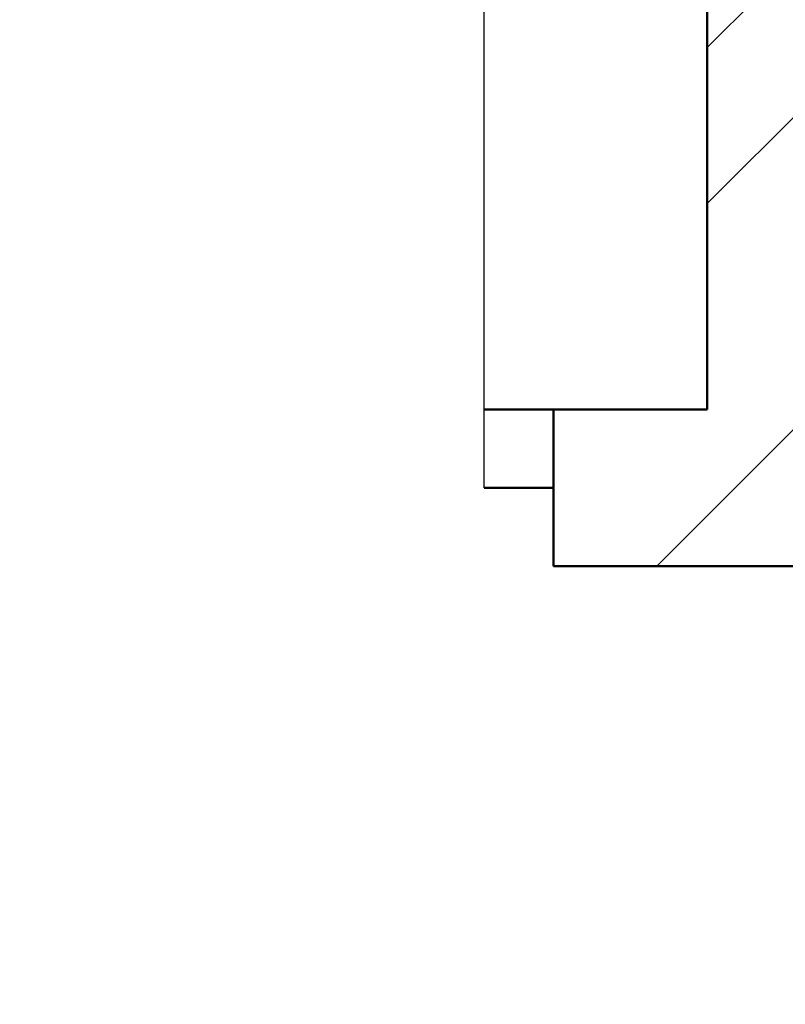
# Model space of a CAD drawing. Units: inches. Extents: x 1901 to 2863, y 888 to 2433.
# Tile 75 of 91: x 2586 to 2608, y 2066 to 2094. Entities that reach past the tile are written whole.
import ezdxf

# ---------------------------------------------------------------- set-up
doc = ezdxf.new("R2010")
doc.units = ezdxf.units.IN
for name, color, linetype, lineweight in [('A-DOOR', 4, 'Continuous', 25), ('A-WALL', 7, 'Continuous', 50), ('A-WALL-PATT', 8, 'Continuous', 13)]:
    doc.layers.add(name, color=color, linetype=linetype, lineweight=lineweight)

# ---------------------------------------------------------------- blocks, each defined once
blk = doc.blocks.new('DOOR-27')
blk.add_line((26.814, -0.016), (26.814, 35.984))
blk.add_arc((26.814, 9.122), 26.862, 90, 199.8893)

msp = doc.modelspace()

# ---------------------------------------------------------------- hatches: boundary and pattern name
at = {"layer": 'A-WALL-PATT'}
h = msp.add_hatch(dxfattribs=at)
h.set_pattern_fill('ANSI32', color=256)
h.paths.add_polyline_path([(2192.501, 2274.134), (2141.264, 2274.134), (2141.264, 2269.634), (2192.501, 2269.634)])
h.paths.add_polyline_path([(2259.926, 2274.134), (2216.501, 2274.134), (2216.501, 2269.634), (2255.426, 2269.634), (2255.426, 2214.634), (2250.809, 2214.634), (2250.809, 2210.134), (2259.926, 2210.134), (2259.926, 2215.134), (2271.756, 2215.134), (2271.756, 2217.384), (2271.756, 2219.634), (2259.926, 2219.634)])
h.paths.add_polyline_path([(2171.426, 2269.634), (2166.926, 2269.634), (2166.926, 2219.634), (2121.238, 2219.634), (2121.238, 2215.134), (2166.926, 2215.134), (2166.926, 2083.134), (2161.807, 2083.134), (2161.807, 2078.634), (2171.426, 2078.634), (2176.996, 2078.634), (2176.996, 2080.884), (2176.996, 2083.134), (2171.426, 2083.134), (2171.426, 2210.134), (2230.912, 2210.134), (2230.912, 2212.384), (2230.912, 2214.634), (2171.426, 2214.634)])
h.paths.add_polyline_path([(2117.264, 2274.134), (2089.426, 2274.134), (2089.426, 2219.634), (2081.136, 2219.634), (2081.136, 2215.134), (2089.426, 2215.134), (2098.004, 2215.134), (2098.004, 2217.384), (2098.004, 2219.634), (2093.926, 2219.634), (2093.926, 2269.634), (2117.264, 2269.634), (2117.264, 2271.884)])
h.paths.add_polyline_path([(2343.426, 2219.634), (2329.295, 2219.634), (2329.295, 2215.134), (2338.926, 2215.134), (2338.926, 2184.739), (2343.426, 2184.739)])
h.paths.add_polyline_path([(2338.926, 2083.134), (2329.295, 2083.134), (2208.966, 2083.134), (2208.966, 2078.634), (2338.926, 2078.634)])
h.paths.add_polyline_path([(2343.426, 2136.739), (2338.926, 2136.739), (2338.926, 1872.634), (2343.426, 1872.634)])
h.paths.add_polyline_path([(2343.426, 1863.634), (2397.68, 1863.634), (2397.68, 1821.634), (2384.138, 1821.634), (2384.138, 1812.634), (2418.33, 1812.634), (2418.33, 1817.134), (2418.33, 1821.634), (2406.68, 1821.634), (2406.68, 1863.634), (2459.499, 1863.634), (2459.499, 1821.634), (2447.138, 1821.634), (2447.138, 1812.634), (2459.499, 1812.634), (2468.499, 1812.634), (2468.499, 1872.634), (2394.426, 1872.634), (2334.426, 1872.634), (2334.426, 1812.634), (2343.426, 1812.634), (2353.251, 1812.634), (2353.251, 1821.634), (2343.426, 1821.634)])
h.paths.add_polyline_path([(2510.014, 1872.634), (2468.499, 1872.634), (2468.499, 1868.134), (2510.014, 1868.134)])
h.paths.add_polyline_path([(2514.009, 1817.134), (2468.499, 1817.134), (2468.499, 1812.634), (2482.114, 1812.634), (2482.114, 1800.606), (2486.614, 1800.606), (2486.614, 1812.634), (2514.009, 1812.634)])
h.paths.add_polyline_path([(2299.247, 1814.884), (2299.247, 1817.134), (2295.926, 1817.134), (2295.926, 1854.169), (2293.676, 1854.169), (2291.426, 1854.169), (2291.426, 1817.134), (2266.109, 1817.134), (2266.109, 1812.634), (2299.247, 1812.634)])
h.paths.add_polyline_path([(2218.109, 1817.134), (2206.46, 1817.134), (2171.426, 1817.134), (2171.426, 1949.134), (2190.1, 1949.134), (2190.1, 1953.634), (2163.468, 1953.634), (2163.468, 1949.134), (2166.926, 1949.134), (2166.926, 1817.134), (2114.297, 1817.134), (2114.297, 1812.634), (2218.109, 1812.634)])
h.paths.add_polyline_path([(2029.426, 1970.922), (2024.926, 1970.922), (2024.926, 1912.717), (2029.426, 1912.717)])
h.paths.add_polyline_path([(2132.297, 1953.634), (2113.926, 1953.634), (2113.926, 1975.888), (2111.676, 1975.888), (2109.426, 1975.888), (2109.426, 1953.634), (2029.426, 1953.634), (2029.426, 1949.134), (2132.297, 1949.134)])
h.paths.add_polyline_path([(2029.426, 1853.606), (2029.31, 1853.606), (2029.31, 1853.606), (2029.426, 1853.606), (2029.426, 1864.717), (2024.926, 1864.717), (2024.926, 1812.634), (2066.297, 1812.634), (2066.297, 1814.884), (2066.297, 1817.134), (2029.426, 1817.134)])
h.paths.add_polyline_path([(2122.926, 2010.088), (2120.676, 2010.088), (2118.426, 2010.088), (2118.426, 2006.134), (2029.426, 2006.134), (2029.426, 2001.634), (2109.426, 2001.634), (2109.426, 1998.041), (2113.926, 1998.041), (2113.926, 2001.634), (2122.926, 2001.634)])
h.paths.add_polyline_path([(2029.426, 2031.376), (2024.926, 2031.376), (2024.926, 1994.922), (2027.176, 1994.922), (2029.426, 1994.922)])
h.paths.add_polyline_path([(2029.426, 2136.739), (2024.926, 2136.739), (2024.926, 2067.376), (2027.176, 2067.376), (2029.426, 2067.376)])
h.paths.add_polyline_path([(2125.618, 2083.134), (2029.426, 2083.134), (2029.426, 2078.634), (2118.426, 2078.634), (2118.426, 2030.715), (2122.926, 2030.715), (2122.926, 2078.634), (2125.618, 2078.634)])
h.paths.add_polyline_path([(2029.426, 2215.134), (2040.468, 2215.134), (2040.468, 2217.384), (2040.468, 2219.634), (2024.926, 2219.634), (2024.926, 2184.739), (2029.426, 2184.739), (2029.426, 2187.778)])
h.paths.add_polyline_path([(2686.426, 2274.134), (2659.284, 2274.134), (2659.284, 2269.634), (2681.926, 2269.634), (2681.926, 2219.634), (2676.816, 2219.634), (2676.816, 2215.134), (2681.926, 2215.134), (2697.011, 2215.134), (2697.011, 2217.384), (2697.011, 2219.634), (2686.426, 2219.634)])
h.paths.add_polyline_path([(2609.926, 2269.634), (2635.284, 2269.634), (2635.284, 2274.134), (2571.431, 2274.134), (2571.431, 2269.634), (2605.426, 2269.634), (2605.426, 2214.634), (2549.098, 2214.634), (2549.098, 2210.134), (2605.426, 2210.134), (2605.426, 2083.134), (2601.014, 2083.134), (2601.014, 2080.884), (2601.014, 2078.634), (2609.926, 2078.634), (2616.162, 2078.634), (2616.162, 2080.884), (2616.162, 2083.134), (2609.926, 2083.134), (2609.926, 2215.134), (2651.465, 2215.134), (2651.465, 2217.384), (2651.465, 2219.634), (2609.926, 2219.634)])
h.paths.add_polyline_path([(2521.426, 2269.634), (2547.431, 2269.634), (2547.431, 2271.884), (2547.431, 2274.134), (2516.926, 2274.134), (2516.926, 2219.634), (2506.41, 2219.634), (2506.41, 2215.134), (2516.926, 2215.134), (2516.926, 2210.134), (2525.402, 2210.134), (2525.402, 2212.384), (2525.402, 2214.634), (2521.426, 2214.634)])
h.paths.add_polyline_path([(2456.011, 2219.634), (2439.426, 2219.634), (2439.426, 2187.888), (2443.926, 2187.888), (2443.926, 2215.134), (2456.011, 2215.134)])
h.paths.add_polyline_path([(2752.926, 2219.634), (2739.485, 2219.634), (2739.485, 2215.134), (2748.426, 2215.134), (2748.426, 2187.888), (2752.926, 2187.888)])
h.paths.add_polyline_path([(2752.926, 2139.888), (2748.426, 2139.888), (2748.426, 2083.134), (2648.416, 2083.134), (2648.416, 2078.634), (2654.926, 2078.634), (2654.926, 2039.437), (2659.426, 2039.437), (2659.426, 2078.634), (2748.426, 2078.634), (2748.426, 2063.429), (2752.926, 2063.429)])
h.paths.add_polyline_path([(2752.926, 2010.634), (2659.426, 2010.634), (2659.426, 2015.652), (2654.926, 2015.652), (2654.926, 2010.634), (2605.426, 2010.634), (2605.426, 1920.967), (2609.926, 1920.967), (2609.926, 2006.134), (2748.426, 2006.134), (2748.426, 1982.466), (2752.926, 1982.466)])
h.paths.add_polyline_path([(2752.926, 2027.429), (2748.426, 2027.429), (2748.426, 2010.634), (2752.926, 2010.634)])
h.paths.add_polyline_path([(2748.426, 1886.134), (2609.926, 1886.134), (2609.926, 1889.719), (2605.426, 1889.719), (2605.426, 1861.262), (2609.926, 1861.262), (2609.926, 1881.634), (2748.426, 1881.634)])
h.paths.add_polyline_path([(2456.855, 2228.831), (2498.401, 2228.831), (2498.401, 2247.488), (2456.855, 2247.488)], flags=9)
h.paths.add_polyline_path([(2038.602, 2237.418), (2080.174, 2237.418), (2080.174, 2256.075), (2038.602, 2256.075)], flags=9)
h.paths.add_polyline_path([(2292.009, 1062.394), (2539.932, 1062.394), (2539.932, 1099.487), (2292.009, 1099.487)], flags=9)
h.paths.add_polyline_path([(2424.91, 1832.253), (2448.513, 1832.253), (2448.513, 1846.678), (2424.91, 1846.678)], flags=25)
h.paths.add_polyline_path([(2359.076, 1832.253), (2382.678, 1832.253), (2382.678, 1846.678), (2359.076, 1846.678)], flags=25)
h.paths.add_polyline_path([(2352.899, 1684.802), (2367.543, 1684.802), (2367.543, 1697.167), (2352.899, 1697.167)], flags=9)
h.paths.add_polyline_path([(2079.288, 1755.826), (2169.024, 1755.826), (2169.024, 1774.372), (2079.288, 1774.372)], flags=9)
h.paths.add_polyline_path([(2404.09, 1373.857), (2404.09, 1463.593), (2385.544, 1463.593), (2385.544, 1373.857)], flags=9)
h.paths.add_polyline_path([(2268.091, 2236.371), (2309.636, 2236.371), (2309.636, 2255.028), (2268.091, 2255.028)], flags=9)
h.paths.add_polyline_path([(2575.96, 1700.951), (2665.696, 1700.951), (2665.696, 1719.498), (2575.96, 1719.498)], flags=9)
h.paths.add_polyline_path([(2302.962, 1878.474), (2329.524, 1878.474), (2329.524, 1888.777), (2302.962, 1888.777)], flags=9)
h.paths.add_polyline_path([(2097.415, 2240.576), (2126.573, 2240.576), (2126.573, 2259.233), (2097.415, 2259.233)], flags=9)
h.paths.add_polyline_path([(2208.725, 2246.124), (2237.882, 2246.124), (2237.882, 2264.781), (2208.725, 2264.781)], flags=9)
h.paths.add_polyline_path([(2038.147, 1925.958), (2076.987, 1925.958), (2076.987, 1944.615), (2038.147, 1944.615)], flags=9)
h.paths.add_polyline_path([(2239.144, 1926.672), (2288.465, 1926.672), (2288.465, 1945.329), (2239.144, 1945.329)], flags=9)
h.paths.add_polyline_path([(2175.429, 2007.33), (2212.356, 2007.33), (2212.356, 2025.987), (2175.429, 2025.987)], flags=9)
h.paths.add_polyline_path([(2225.034, 2091.794), (2263.875, 2091.794), (2263.875, 2110.451), (2225.034, 2110.451)], flags=9)
h.paths.add_polyline_path([(2035.398, 2098.478), (2074.238, 2098.478), (2074.238, 2117.135), (2035.398, 2117.135)], flags=9)
h.paths.add_polyline_path([(2050.102, 2029.209), (2083.26, 2029.209), (2083.26, 2047.866), (2050.102, 2047.866)], flags=9)
h.paths.add_polyline_path([(2069.677, 1956.719), (2098.835, 1956.719), (2098.835, 1975.376), (2069.677, 1975.376)], flags=25)
h.paths.add_polyline_path([(2328.62, 1753.336), (2361.663, 1753.336), (2361.663, 1771.993), (2328.62, 1771.993)], flags=9)
h.paths.add_polyline_path([(2395.162, 2060.888), (2395.162, 2140.654), (2378.676, 2140.654), (2378.676, 2060.888)], flags=9)
h.paths.add_polyline_path([(2463.728, 2059.02), (2492.886, 2059.02), (2492.886, 2077.677), (2463.728, 2077.677)], flags=9)
h.paths.add_polyline_path([(2458.027, 2181.536), (2496.868, 2181.536), (2496.868, 2200.194), (2458.027, 2200.194)], flags=9)
h.paths.add_polyline_path([(2527.577, 2243.074), (2556.735, 2243.074), (2556.735, 2261.731), (2527.577, 2261.731)], flags=9)
h.paths.add_polyline_path([(2694.461, 2232.767), (2736.033, 2232.767), (2736.033, 2251.425), (2694.461, 2251.425)], flags=9)
h.paths.add_polyline_path([(2637.821, 2249.225), (2666.979, 2249.225), (2666.979, 2267.882), (2637.821, 2267.882)], flags=9)
h.paths.add_polyline_path([(2623.687, 2183.541), (2662.528, 2183.541), (2662.528, 2202.199), (2623.687, 2202.199)], flags=9)
h.paths.add_polyline_path([(2691.965, 2021.5), (2725.124, 2021.5), (2725.124, 2040.157), (2691.965, 2040.157)], flags=9)
h.paths.add_polyline_path([(2621.043, 1975.912), (2662.335, 1975.912), (2662.335, 1994.569), (2621.043, 1994.569)], flags=25)
h.paths.add_polyline_path([(2479.032, 1927.62), (2519.844, 1927.62), (2519.844, 1946.277), (2479.032, 1946.277)], flags=9)
h.paths.add_polyline_path([(2670.941, 1849.076), (2716.005, 1849.076), (2716.005, 1867.734), (2670.941, 1867.734)], flags=9)
h.paths.add_polyline_path([(2523.613, 1782.956), (2550.175, 1782.956), (2550.175, 1793.26), (2523.613, 1793.26)], flags=9)
h.paths.add_polyline_path([(2450.841, 1207.331), (2492.386, 1207.331), (2492.386, 1225.989), (2450.841, 1225.989)], flags=9)
h.paths.add_polyline_path([(2527.751, 1203.841), (2556.908, 1203.841), (2556.908, 1222.499), (2527.751, 1222.499)], flags=9)
h.paths.add_polyline_path([(2639.111, 1207.2), (2668.268, 1207.2), (2668.268, 1225.857), (2639.111, 1225.857)], flags=9)
h.paths.add_polyline_path([(2692.594, 1218.965), (2734.167, 1218.965), (2734.167, 1237.623), (2692.594, 1237.623)], flags=9)
h.paths.add_polyline_path([(2669.266, 1366.329), (2708.106, 1366.329), (2708.106, 1384.987), (2669.266, 1384.987)], flags=9)
h.paths.add_polyline_path([(2463.313, 1358.031), (2502.153, 1358.031), (2502.153, 1376.688), (2463.313, 1376.688)], flags=9)
h.paths.add_polyline_path([(2494.725, 1449.963), (2531.652, 1449.963), (2531.652, 1468.62), (2494.725, 1468.62)], flags=9)
h.paths.add_polyline_path([(2675.565, 1422.157), (2708.724, 1422.157), (2708.724, 1440.815), (2675.565, 1440.815)], flags=9)
h.paths.add_polyline_path([(2685.634, 1493.891), (2714.792, 1493.891), (2714.792, 1512.548), (2685.634, 1512.548)], flags=9)
h.paths.add_polyline_path([(2686.805, 1529.913), (2725.645, 1529.913), (2725.645, 1548.57), (2686.805, 1548.57)], flags=9)
h.paths.add_polyline_path([(2503.651, 1537.991), (2552.972, 1537.991), (2552.972, 1556.648), (2503.651, 1556.648)], flags=9)
h.paths.add_polyline_path([(2291.713, 1643.504), (2318.275, 1643.504), (2318.275, 1653.807), (2291.713, 1653.807)], flags=9)
h.paths.add_polyline_path([(2450.626, 1610.52), (2477.189, 1610.52), (2477.189, 1620.824), (2450.626, 1620.824)], flags=9)
h.paths.add_polyline_path([(2359.985, 1551.814), (2422.253, 1551.814), (2422.253, 1562.117), (2359.985, 1562.117)], flags=9)
h.paths.add_polyline_path([(2280.106, 1249.006), (2321.651, 1249.006), (2321.651, 1267.663), (2280.106, 1267.663)], flags=9)
h.paths.add_polyline_path([(2164.057, 1274.232), (2193.215, 1274.232), (2193.215, 1292.889), (2164.057, 1292.889)], flags=9)
h.paths.add_polyline_path([(2118.21, 1277.694), (2151.252, 1277.694), (2151.252, 1296.351), (2118.21, 1296.351)], flags=9)
h.paths.add_polyline_path([(2031.946, 1268.529), (2073.519, 1268.529), (2073.519, 1287.187), (2031.946, 1287.187)], flags=9)
h.paths.add_polyline_path([(2050.199, 1409.079), (2089.04, 1409.079), (2089.04, 1427.736), (2050.199, 1427.736)], flags=9)
h.paths.add_polyline_path([(2243.743, 1421.032), (2282.584, 1421.032), (2282.584, 1439.689), (2243.743, 1439.689)], flags=9)
h.paths.add_polyline_path([(2190.746, 1509.769), (2231.558, 1509.769), (2231.558, 1528.426), (2190.746, 1528.426)], flags=9)
h.paths.add_polyline_path([(2058.392, 1475.415), (2091.55, 1475.415), (2091.55, 1494.073), (2058.392, 1494.073)], flags=9)
h.paths.add_polyline_path([(2062.447, 1553.09), (2091.605, 1553.09), (2091.605, 1571.747), (2062.447, 1571.747)], flags=9)
h.paths.add_polyline_path([(2219.524, 1590.365), (2266.147, 1590.365), (2266.147, 1609.022), (2219.524, 1609.022)], flags=9)
h.paths.add_polyline_path([(2041.072, 1584.188), (2079.912, 1584.188), (2079.912, 1602.845), (2041.072, 1602.845)], flags=9)

# ---------------------------------------------------------------- linework, layer by layer
at = {"layer": 'A-WALL'}
for p, q in [((2605.426, 2210.134), (2605.426, 2083.134)), ((2599.014, 2083.134), (2605.426, 2083.134)), ((2601.014, 2078.634), (2601.014, 2083.134)), ((2601.014, 2083.134), (2601.014, 2080.884)), ((2601.014, 2080.884), (2599.014, 2080.884)), ((2601.014, 2078.634), (2609.926, 2078.634))]:
    msp.add_line(p, q, dxfattribs=at)

# ---------------------------------------------------------------- block references
at = {"layer": 'A-DOOR'}
msp.add_blockref('DOOR-27', (2572.2, 2080.9), dxfattribs=at)

doc.saveas('drawing.dxf')
